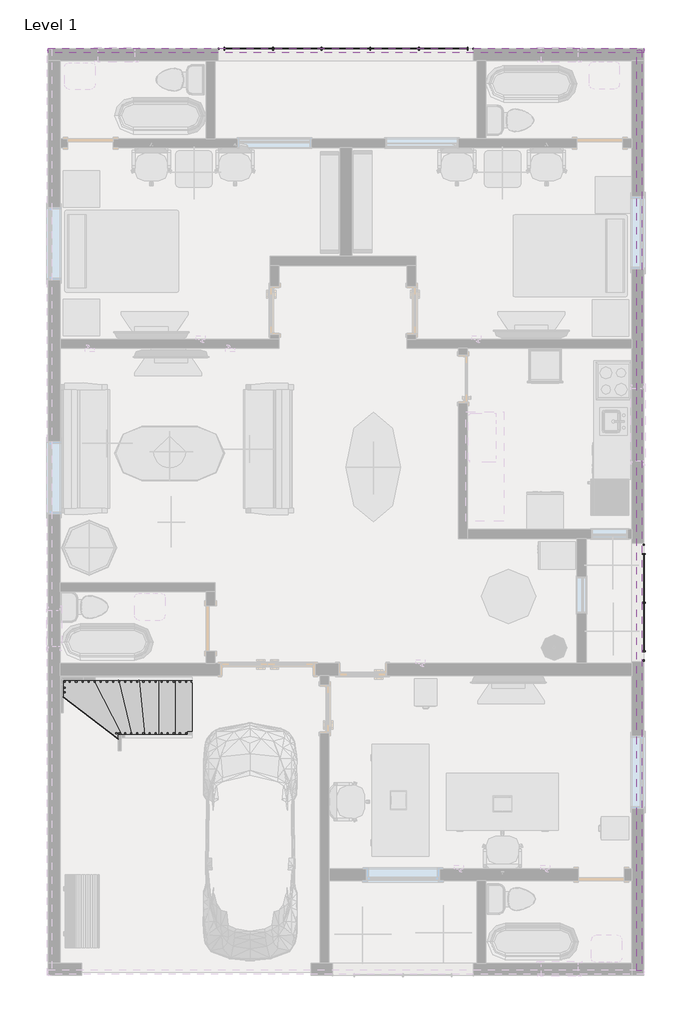
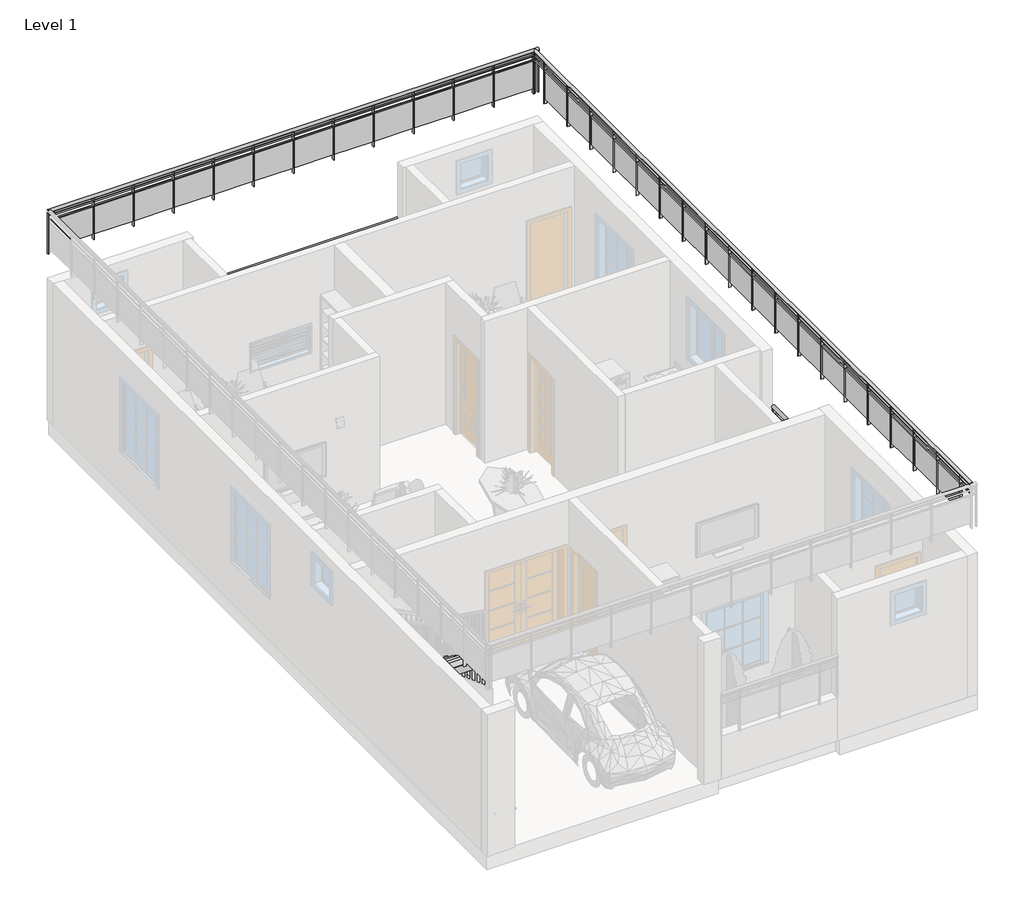
# One storey, part 4 of 5: 4 railings, 1 stair flight.
"""IFC4 building model written with IfcOpenShell, lengths in millimetres."""

from ifc_helpers import new_model, si_unit, point, frame, origin, place, context, project, spatial, polyline, ellipse_curve, trimmed, outline, extrude, transform, mapped, element, save
from ifc_brep_helpers import plane_surface, extruded_surface, advanced_brep
from components import stair_flight_393df7a1

model = new_model("IFC4")

# Units and contexts
model_context = context("Model", 3, world=origin())
ifc_project = project(units=[si_unit("LENGTHUNIT", "METRE", prefix="MILLI")], contexts=[model_context])

# Site, building, storey
site = spatial("IfcSite", under=ifc_project)
building = spatial("IfcBuilding", under=site)
storey = spatial("IfcBuildingStorey", under=building, Name="Level 1", Elevation=0.0)

# Railings
placement = place(None, origin())
element("IfcRailing", 1, ObjectType="Glass Panel - Bottom Fill", at=placement, inside=storey, context=model_context, shape_type="SolidModel", body=[
    advanced_brep(
    [(-4454.3957152, 16105.8691167, 1828.8), (-4454.3957152, 16029.6691167, 1828.8), (-187.1957152, 16105.8691167, 1828.8), (-187.1957152, 16029.6691167, 1828.8)],
    [
        (0, 1, ellipse_curve(frame((-4454.3957152, 16067.7691167, 1828.8), z_axis=(-1.0, 0.0, 0.0), x_axis=(0.0, -1.0, 0.0)), 38.1, 28.575)),
        (1, 0, ellipse_curve(frame((-4454.3957152, 16067.7691167, 1828.8), z_axis=(-1.0, 0.0, 0.0), x_axis=(0.0, -1.0, 0.0)), 38.1, 28.575)),
        (2, 3, ellipse_curve(frame((-187.1957152, 16067.7691167, 1828.8), z_axis=(1.0, 0.0, 0.0), x_axis=(0.0, -1.0, 0.0)), 38.1, 28.575)),
        (3, 2, ellipse_curve(frame((-187.1957152, 16067.7691167, 1828.8), z_axis=(1.0, 0.0, 0.0), x_axis=(0.0, -1.0, 0.0)), 38.1, 28.575)),
        (0, 2),
        (3, 1),
    ],
    [
        plane_surface(frame((-4454.3957152, 16067.7691167, 1828.8), z_axis=(-1.0, 0.0, 0.0), x_axis=(0.0, 1.0, 0.0))),
        plane_surface(frame((-187.1957152, 16067.7691167, 1828.8), z_axis=(1.0, 0.0, 0.0), x_axis=(0.0, 1.0, 0.0))),
        extruded_surface(trimmed(ellipse_curve(frame((-187.1957152, 16067.7691167, 1828.8), z_axis=(-1.0, 0.0, 0.0), x_axis=(0.0, -1.0, 0.0)), 38.1, 28.575), [point((-187.1957152, 16105.8691167, 1828.8))], [point((-187.1957152, 16029.6691167, 1828.8))], True, "CARTESIAN"), (-4267.200000000001, 0.0, 0.0), 4267.200000000001),
        extruded_surface(trimmed(ellipse_curve(frame((-187.1957152, 16067.7691167, 1828.8), z_axis=(-1.0, 0.0, 0.0), x_axis=(0.0, -1.0, 0.0)), 38.1, 28.575), [point((-187.1957152, 16029.6691167, 1828.8))], [point((-187.1957152, 16105.8691167, 1828.8))], True, "CARTESIAN"), (-4267.200000000001, 0.0, 0.0), 4267.200000000001),
    ],
    [
        (0, [[1, 2]]),
        (1, [[3, 4]]),
        (2, [[-1, 5, -4, 6]]),
        (3, [[-2, -6, -3, -5]]),
    ],
),
    extrude(outline(polyline([(-4454.3957152, 16055.0691167), (-4454.3957152, 16080.4691167), (-187.1957152, 16080.4691167), (-187.1957152, 16055.0691167), (-4454.3957152, 16055.0691167)])), frame((0.0, 0.0, 1714.5), z_axis=(0.0, 0.0, 1.0), x_axis=(1.0, 0.0, 0.0)), (0.0, 0.0, 1.0), 25.4),
    extrude(outline(polyline([(-4454.3957152, 16055.0691167), (-4454.3957152, 16080.4691167), (-187.1957152, 16080.4691167), (-187.1957152, 16055.0691167), (-4454.3957152, 16055.0691167)])), frame((0.0, 0.0, 1612.9), z_axis=(0.0, 0.0, 1.0), x_axis=(1.0, 0.0, 0.0)), (0.0, 0.0, 1.0), 25.4),
    extrude(outline(polyline([(-295.1457152, 16042.3691167), (-295.1457152, 16093.1691167), (-282.4457152, 16093.1691167), (-282.4457152, 16042.3691167), (-295.1457152, 16042.3691167)])), frame((0.0, 0.0, 914.4), z_axis=(0.0, 0.0, 1.0), x_axis=(1.0, 0.0, 0.0)), (0.0, 0.0, 1.0), 885.6788223),
    extrude(outline(polyline([(-1101.5957152, 16074.3042737), (-288.7957152, 16074.3042737), (-288.7957152, 16067.9542737), (-1101.5957152, 16067.9542737), (-1101.5957152, 16074.3042737)])), frame((0.0, 0.0, 1016.0), z_axis=(0.0, 0.0, 1.0), x_axis=(1.0, 0.0, 0.0)), (0.0, 0.0, 1.0), 596.9),
    extrude(outline(polyline([(-1107.9457152, 16042.3691167), (-1107.9457152, 16093.1691167), (-1095.2457152, 16093.1691167), (-1095.2457152, 16042.3691167), (-1107.9457152, 16042.3691167)])), frame((0.0, 0.0, 914.4), z_axis=(0.0, 0.0, 1.0), x_axis=(1.0, 0.0, 0.0)), (0.0, 0.0, 1.0), 885.6788223),
    extrude(outline(polyline([(-1914.3957152, 16074.3042737), (-1101.5957152, 16074.3042737), (-1101.5957152, 16067.9542737), (-1914.3957152, 16067.9542737), (-1914.3957152, 16074.3042737)])), frame((0.0, 0.0, 1016.0), z_axis=(0.0, 0.0, 1.0), x_axis=(1.0, 0.0, 0.0)), (0.0, 0.0, 1.0), 596.9),
    extrude(outline(polyline([(-1920.7457152, 16042.3691167), (-1920.7457152, 16093.1691167), (-1908.0457152, 16093.1691167), (-1908.0457152, 16042.3691167), (-1920.7457152, 16042.3691167)])), frame((0.0, 0.0, 914.4), z_axis=(0.0, 0.0, 1.0), x_axis=(1.0, 0.0, 0.0)), (0.0, 0.0, 1.0), 885.6788223),
    extrude(outline(polyline([(-2727.1957152, 16074.3042737), (-1914.3957152, 16074.3042737), (-1914.3957152, 16067.9542737), (-2727.1957152, 16067.9542737), (-2727.1957152, 16074.3042737)])), frame((0.0, 0.0, 1016.0), z_axis=(0.0, 0.0, 1.0), x_axis=(1.0, 0.0, 0.0)), (0.0, 0.0, 1.0), 596.9),
    extrude(outline(polyline([(-2733.5457152, 16042.3691167), (-2733.5457152, 16093.1691167), (-2720.8457152, 16093.1691167), (-2720.8457152, 16042.3691167), (-2733.5457152, 16042.3691167)])), frame((0.0, 0.0, 914.4), z_axis=(0.0, 0.0, 1.0), x_axis=(1.0, 0.0, 0.0)), (0.0, 0.0, 1.0), 885.6788223),
    extrude(outline(polyline([(-3539.9957152, 16074.3042737), (-2727.1957152, 16074.3042737), (-2727.1957152, 16067.9542737), (-3539.9957152, 16067.9542737), (-3539.9957152, 16074.3042737)])), frame((0.0, 0.0, 1016.0), z_axis=(0.0, 0.0, 1.0), x_axis=(1.0, 0.0, 0.0)), (0.0, 0.0, 1.0), 596.9),
    extrude(outline(polyline([(-3546.3457152, 16042.3691167), (-3546.3457152, 16093.1691167), (-3533.6457152, 16093.1691167), (-3533.6457152, 16042.3691167), (-3546.3457152, 16042.3691167)])), frame((0.0, 0.0, 914.4), z_axis=(0.0, 0.0, 1.0), x_axis=(1.0, 0.0, 0.0)), (0.0, 0.0, 1.0), 885.6788223),
    extrude(outline(polyline([(-4352.7957152, 16074.3042737), (-3539.9957152, 16074.3042737), (-3539.9957152, 16067.9542737), (-4352.7957152, 16067.9542737), (-4352.7957152, 16074.3042737)])), frame((0.0, 0.0, 1016.0), z_axis=(0.0, 0.0, 1.0), x_axis=(1.0, 0.0, 0.0)), (0.0, 0.0, 1.0), 596.9),
    extrude(outline(polyline([(-4359.1457152, 16042.3691167), (-4359.1457152, 16093.1691167), (-4346.4457152, 16093.1691167), (-4346.4457152, 16042.3691167), (-4359.1457152, 16042.3691167)])), frame((0.0, 0.0, 914.4), z_axis=(0.0, 0.0, 1.0), x_axis=(1.0, 0.0, 0.0)), (0.0, 0.0, 1.0), 885.6788223),
    extrude(outline(polyline([(-199.8957152, 16058.2441167), (-199.8957152, 16077.2941167), (-180.8457152, 16077.2941167), (-180.8457152, 16058.2441167), (-199.8957152, 16058.2441167)])), frame((0.0, 0.0, 914.4), z_axis=(0.0, 0.0, 1.0), x_axis=(1.0, 0.0, 0.0)), (0.0, 0.0, 1.0), 885.6788223),
    extrude(outline(polyline([(-4460.7457152, 16058.2441167), (-4460.7457152, 16077.2941167), (-4441.6957152, 16077.2941167), (-4441.6957152, 16058.2441167), (-4460.7457152, 16058.2441167)])), frame((0.0, 0.0, 914.4), z_axis=(0.0, 0.0, 1.0), x_axis=(1.0, 0.0, 0.0)), (0.0, 0.0, 1.0), 885.6788223),
])
element("IfcRailing", 2, ObjectType="Glass Panel - Bottom Fill", at=placement, inside=storey, context=model_context, shape_type="SolidModel", body=[
    advanced_brep(
    [(2695.7042848, 7787.3691167, 1828.8), (2619.5042848, 7787.3691167, 1828.8), (2695.7042848, 5850.6191167, 1828.8), (2619.5042848, 5850.6191167, 1828.8)],
    [
        (0, 1, ellipse_curve(frame((2657.6042848, 7787.3691167, 1828.8), z_axis=(0.0, 1.0, 0.0), x_axis=(-1.0, 0.0, 0.0)), 38.1, 28.575)),
        (1, 0, ellipse_curve(frame((2657.6042848, 7787.3691167, 1828.8), z_axis=(0.0, 1.0, 0.0), x_axis=(-1.0, 0.0, 0.0)), 38.1, 28.575)),
        (2, 3, ellipse_curve(frame((2657.6042848, 5850.6191167, 1828.8), z_axis=(0.0, -1.0, 0.0), x_axis=(-1.0, 0.0, 0.0)), 38.1, 28.575)),
        (3, 2, ellipse_curve(frame((2657.6042848, 5850.6191167, 1828.8), z_axis=(0.0, -1.0, 0.0), x_axis=(-1.0, 0.0, 0.0)), 38.1, 28.575)),
        (0, 2),
        (3, 1),
    ],
    [
        plane_surface(frame((2657.6042848, 7787.3691167, 1828.8), z_axis=(0.0, 1.0, 0.0), x_axis=(0.0, 0.0, -1.0))),
        plane_surface(frame((2657.6042848, 5850.6191167, 1828.8), z_axis=(0.0, -1.0, 0.0), x_axis=(0.0, 0.0, -1.0))),
        extruded_surface(trimmed(ellipse_curve(frame((2657.6042848, 5850.6191167, 1828.8), z_axis=(0.0, 1.0, 0.0), x_axis=(-1.0, 0.0, 0.0)), 38.1, 28.575), [point((2695.7042848, 5850.6191167, 1828.8))], [point((2619.5042848, 5850.6191167, 1828.8))], True, "CARTESIAN"), (0.0, 1936.75, 0.0), 1936.75),
        extruded_surface(trimmed(ellipse_curve(frame((2657.6042848, 5850.6191167, 1828.8), z_axis=(0.0, 1.0, 0.0), x_axis=(-1.0, 0.0, 0.0)), 38.1, 28.575), [point((2619.5042848, 5850.6191167, 1828.8))], [point((2695.7042848, 5850.6191167, 1828.8))], True, "CARTESIAN"), (0.0, 1936.75, 0.0), 1936.75),
    ],
    [
        (0, [[1, 2]]),
        (1, [[3, 4]]),
        (2, [[-1, 5, -4, 6]]),
        (3, [[-2, -6, -3, -5]]),
    ],
),
    extrude(outline(polyline([(2644.9042848, 7787.3691167), (2670.3042848, 7787.3691167), (2670.3042848, 5850.6191167), (2644.9042848, 5850.6191167), (2644.9042848, 7787.3691167)])), frame((0.0, 0.0, 1714.5), z_axis=(0.0, 0.0, 1.0), x_axis=(1.0, 0.0, 0.0)), (0.0, 0.0, 1.0), 25.4),
    extrude(outline(polyline([(2644.9042848, 7787.3691167), (2670.3042848, 7787.3691167), (2670.3042848, 5850.6191167), (2644.9042848, 5850.6191167), (2644.9042848, 7787.3691167)])), frame((0.0, 0.0, 1612.9), z_axis=(0.0, 0.0, 1.0), x_axis=(1.0, 0.0, 0.0)), (0.0, 0.0, 1.0), 25.4),
    extrude(outline(polyline([(2632.2042848, 6012.5441167), (2683.0042848, 6012.5441167), (2683.0042848, 5999.8441167), (2632.2042848, 5999.8441167), (2632.2042848, 6012.5441167)])), frame((0.0, 0.0, 914.4), z_axis=(0.0, 0.0, 1.0), x_axis=(1.0, 0.0, 0.0)), (0.0, 0.0, 1.0), 885.6788223),
    extrude(outline(polyline([(2664.1394419, 6818.9941167), (2664.1394419, 6006.1941167), (2657.7894419, 6006.1941167), (2657.7894419, 6818.9941167), (2664.1394419, 6818.9941167)])), frame((0.0, 0.0, 1016.0), z_axis=(0.0, 0.0, 1.0), x_axis=(1.0, 0.0, 0.0)), (0.0, 0.0, 1.0), 596.9),
    extrude(outline(polyline([(2632.2042848, 6825.3441167), (2683.0042848, 6825.3441167), (2683.0042848, 6812.6441167), (2632.2042848, 6812.6441167), (2632.2042848, 6825.3441167)])), frame((0.0, 0.0, 914.4), z_axis=(0.0, 0.0, 1.0), x_axis=(1.0, 0.0, 0.0)), (0.0, 0.0, 1.0), 885.6788223),
    extrude(outline(polyline([(2664.1394419, 7631.7941167), (2664.1394419, 6818.9941167), (2657.7894419, 6818.9941167), (2657.7894419, 7631.7941167), (2664.1394419, 7631.7941167)])), frame((0.0, 0.0, 1016.0), z_axis=(0.0, 0.0, 1.0), x_axis=(1.0, 0.0, 0.0)), (0.0, 0.0, 1.0), 596.9),
    extrude(outline(polyline([(2632.2042848, 7638.1441167), (2683.0042848, 7638.1441167), (2683.0042848, 7625.4441167), (2632.2042848, 7625.4441167), (2632.2042848, 7638.1441167)])), frame((0.0, 0.0, 914.4), z_axis=(0.0, 0.0, 1.0), x_axis=(1.0, 0.0, 0.0)), (0.0, 0.0, 1.0), 885.6788223),
    extrude(outline(polyline([(2648.0792848, 5863.3191167), (2667.1292848, 5863.3191167), (2667.1292848, 5844.2691167), (2648.0792848, 5844.2691167), (2648.0792848, 5863.3191167)])), frame((0.0, 0.0, 914.4), z_axis=(0.0, 0.0, 1.0), x_axis=(1.0, 0.0, 0.0)), (0.0, 0.0, 1.0), 885.6788223),
    extrude(outline(polyline([(2648.0792848, 7793.7191167), (2667.1292848, 7793.7191167), (2667.1292848, 7774.6691167), (2648.0792848, 7774.6691167), (2648.0792848, 7793.7191167)])), frame((0.0, 0.0, 914.4), z_axis=(0.0, 0.0, 1.0), x_axis=(1.0, 0.0, 0.0)), (0.0, 0.0, 1.0), 885.6788223),
])
element("IfcRailing", 3, ObjectType="Glass Panel - Bottom Fill", at=placement, inside=storey, context=model_context, shape_type="SolidModel", body=[
    advanced_brep(
    [(-7299.1957152, 16080.4691167, 4495.8), (-7299.1957152, 16004.2691167, 4495.8), (2657.6042848, 16080.4691167, 4495.8), (2657.6042848, 16004.2691167, 4495.8)],
    [
        (0, 1, ellipse_curve(frame((-7299.1957152, 16042.3691167, 4495.8), z_axis=(-1.0, 0.0, 0.0), x_axis=(0.0, -1.0, 0.0)), 38.1, 28.575)),
        (1, 0, ellipse_curve(frame((-7299.1957152, 16042.3691167, 4495.8), z_axis=(-1.0, 0.0, 0.0), x_axis=(0.0, -1.0, 0.0)), 38.1, 28.575)),
        (2, 3, ellipse_curve(frame((2657.6042848, 16042.3691167, 4495.8), z_axis=(1.0, 0.0, 0.0), x_axis=(0.0, -1.0, 0.0)), 38.1, 28.575)),
        (3, 2, ellipse_curve(frame((2657.6042848, 16042.3691167, 4495.8), z_axis=(1.0, 0.0, 0.0), x_axis=(0.0, -1.0, 0.0)), 38.1, 28.575)),
        (0, 2),
        (3, 1),
    ],
    [
        plane_surface(frame((-7299.1957152, 16042.3691167, 4495.8), z_axis=(-1.0, 0.0, 0.0), x_axis=(0.0, 1.0, 0.0))),
        plane_surface(frame((2657.6042848, 16042.3691167, 4495.8), z_axis=(1.0, 0.0, 0.0), x_axis=(0.0, 1.0, 0.0))),
        extruded_surface(trimmed(ellipse_curve(frame((2657.6042848, 16042.3691167, 4495.8), z_axis=(-1.0, 0.0, 0.0), x_axis=(0.0, -1.0, 0.0)), 38.1, 28.575), [point((2657.6042848, 16080.4691167, 4495.8))], [point((2657.6042848, 16004.2691167, 4495.8))], True, "CARTESIAN"), (-9956.800000000001, 0.0, 0.0), 9956.800000000001),
        extruded_surface(trimmed(ellipse_curve(frame((2657.6042848, 16042.3691167, 4495.8), z_axis=(-1.0, 0.0, 0.0), x_axis=(0.0, -1.0, 0.0)), 38.1, 28.575), [point((2657.6042848, 16004.2691167, 4495.8))], [point((2657.6042848, 16080.4691167, 4495.8))], True, "CARTESIAN"), (-9956.800000000001, 0.0, 0.0), 9956.800000000001),
    ],
    [
        (0, [[1, 2]]),
        (1, [[3, 4]]),
        (2, [[-1, 5, -4, 6]]),
        (3, [[-2, -6, -3, -5]]),
    ],
),
    extrude(outline(polyline([(-7299.1957152, 16029.6691167), (-7299.1957152, 16055.0691167), (2657.6042848, 16055.0691167), (2657.6042848, 16029.6691167), (-7299.1957152, 16029.6691167)])), frame((0.0, 0.0, 4381.5), z_axis=(0.0, 0.0, 1.0), x_axis=(1.0, 0.0, 0.0)), (0.0, 0.0, 1.0), 25.4),
    extrude(outline(polyline([(-7299.1957152, 16029.6691167), (-7299.1957152, 16055.0691167), (2657.6042848, 16055.0691167), (2657.6042848, 16029.6691167), (-7299.1957152, 16029.6691167)])), frame((0.0, 0.0, 4279.9), z_axis=(0.0, 0.0, 1.0), x_axis=(1.0, 0.0, 0.0)), (0.0, 0.0, 1.0), 25.4),
    extrude(outline(polyline([(2549.6542848, 16016.9691167), (2549.6542848, 16067.7691167), (2562.3542848, 16067.7691167), (2562.3542848, 16016.9691167), (2549.6542848, 16016.9691167)])), frame((0.0, 0.0, 3581.4), z_axis=(0.0, 0.0, 1.0), x_axis=(1.0, 0.0, 0.0)), (0.0, 0.0, 1.0), 885.6788223),
    extrude(outline(polyline([(1743.2042848, 16048.9042737), (2556.0042848, 16048.9042737), (2556.0042848, 16042.5542737), (1743.2042848, 16042.5542737), (1743.2042848, 16048.9042737)])), frame((0.0, 0.0, 3683.0), z_axis=(0.0, 0.0, 1.0), x_axis=(1.0, 0.0, 0.0)), (0.0, 0.0, 1.0), 596.9),
    extrude(outline(polyline([(1736.8542848, 16016.9691167), (1736.8542848, 16067.7691167), (1749.5542848, 16067.7691167), (1749.5542848, 16016.9691167), (1736.8542848, 16016.9691167)])), frame((0.0, 0.0, 3581.4), z_axis=(0.0, 0.0, 1.0), x_axis=(1.0, 0.0, 0.0)), (0.0, 0.0, 1.0), 885.6788223),
    extrude(outline(polyline([(930.4042848, 16048.9042737), (1743.2042848, 16048.9042737), (1743.2042848, 16042.5542737), (930.4042848, 16042.5542737), (930.4042848, 16048.9042737)])), frame((0.0, 0.0, 3683.0), z_axis=(0.0, 0.0, 1.0), x_axis=(1.0, 0.0, 0.0)), (0.0, 0.0, 1.0), 596.9),
    extrude(outline(polyline([(924.0542848, 16016.9691167), (924.0542848, 16067.7691167), (936.7542848, 16067.7691167), (936.7542848, 16016.9691167), (924.0542848, 16016.9691167)])), frame((0.0, 0.0, 3581.4), z_axis=(0.0, 0.0, 1.0), x_axis=(1.0, 0.0, 0.0)), (0.0, 0.0, 1.0), 885.6788223),
    extrude(outline(polyline([(117.6042848, 16048.9042737), (930.4042848, 16048.9042737), (930.4042848, 16042.5542737), (117.6042848, 16042.5542737), (117.6042848, 16048.9042737)])), frame((0.0, 0.0, 3683.0), z_axis=(0.0, 0.0, 1.0), x_axis=(1.0, 0.0, 0.0)), (0.0, 0.0, 1.0), 596.9),
    extrude(outline(polyline([(111.2542848, 16016.9691167), (111.2542848, 16067.7691167), (123.9542848, 16067.7691167), (123.9542848, 16016.9691167), (111.2542848, 16016.9691167)])), frame((0.0, 0.0, 3581.4), z_axis=(0.0, 0.0, 1.0), x_axis=(1.0, 0.0, 0.0)), (0.0, 0.0, 1.0), 885.6788223),
    extrude(outline(polyline([(-695.1957152, 16048.9042737), (117.6042848, 16048.9042737), (117.6042848, 16042.5542737), (-695.1957152, 16042.5542737), (-695.1957152, 16048.9042737)])), frame((0.0, 0.0, 3683.0), z_axis=(0.0, 0.0, 1.0), x_axis=(1.0, 0.0, 0.0)), (0.0, 0.0, 1.0), 596.9),
    extrude(outline(polyline([(-701.5457152, 16016.9691167), (-701.5457152, 16067.7691167), (-688.8457152, 16067.7691167), (-688.8457152, 16016.9691167), (-701.5457152, 16016.9691167)])), frame((0.0, 0.0, 3581.4), z_axis=(0.0, 0.0, 1.0), x_axis=(1.0, 0.0, 0.0)), (0.0, 0.0, 1.0), 885.6788223),
    extrude(outline(polyline([(-1507.9957152, 16048.9042737), (-695.1957152, 16048.9042737), (-695.1957152, 16042.5542737), (-1507.9957152, 16042.5542737), (-1507.9957152, 16048.9042737)])), frame((0.0, 0.0, 3683.0), z_axis=(0.0, 0.0, 1.0), x_axis=(1.0, 0.0, 0.0)), (0.0, 0.0, 1.0), 596.9),
    extrude(outline(polyline([(-1514.3457152, 16016.9691167), (-1514.3457152, 16067.7691167), (-1501.6457152, 16067.7691167), (-1501.6457152, 16016.9691167), (-1514.3457152, 16016.9691167)])), frame((0.0, 0.0, 3581.4), z_axis=(0.0, 0.0, 1.0), x_axis=(1.0, 0.0, 0.0)), (0.0, 0.0, 1.0), 885.6788223),
    extrude(outline(polyline([(-2320.7957152, 16048.9042737), (-1507.9957152, 16048.9042737), (-1507.9957152, 16042.5542737), (-2320.7957152, 16042.5542737), (-2320.7957152, 16048.9042737)])), frame((0.0, 0.0, 3683.0), z_axis=(0.0, 0.0, 1.0), x_axis=(1.0, 0.0, 0.0)), (0.0, 0.0, 1.0), 596.9),
    extrude(outline(polyline([(-2327.1457152, 16016.9691167), (-2327.1457152, 16067.7691167), (-2314.4457152, 16067.7691167), (-2314.4457152, 16016.9691167), (-2327.1457152, 16016.9691167)])), frame((0.0, 0.0, 3581.4), z_axis=(0.0, 0.0, 1.0), x_axis=(1.0, 0.0, 0.0)), (0.0, 0.0, 1.0), 885.6788223),
    extrude(outline(polyline([(-3133.5957152, 16048.9042737), (-2320.7957152, 16048.9042737), (-2320.7957152, 16042.5542737), (-3133.5957152, 16042.5542737), (-3133.5957152, 16048.9042737)])), frame((0.0, 0.0, 3683.0), z_axis=(0.0, 0.0, 1.0), x_axis=(1.0, 0.0, 0.0)), (0.0, 0.0, 1.0), 596.9),
    extrude(outline(polyline([(-3139.9457152, 16016.9691167), (-3139.9457152, 16067.7691167), (-3127.2457152, 16067.7691167), (-3127.2457152, 16016.9691167), (-3139.9457152, 16016.9691167)])), frame((0.0, 0.0, 3581.4), z_axis=(0.0, 0.0, 1.0), x_axis=(1.0, 0.0, 0.0)), (0.0, 0.0, 1.0), 885.6788223),
    extrude(outline(polyline([(-3946.3957152, 16048.9042737), (-3133.5957152, 16048.9042737), (-3133.5957152, 16042.5542737), (-3946.3957152, 16042.5542737), (-3946.3957152, 16048.9042737)])), frame((0.0, 0.0, 3683.0), z_axis=(0.0, 0.0, 1.0), x_axis=(1.0, 0.0, 0.0)), (0.0, 0.0, 1.0), 596.9),
    extrude(outline(polyline([(-3952.7457152, 16016.9691167), (-3952.7457152, 16067.7691167), (-3940.0457152, 16067.7691167), (-3940.0457152, 16016.9691167), (-3952.7457152, 16016.9691167)])), frame((0.0, 0.0, 3581.4), z_axis=(0.0, 0.0, 1.0), x_axis=(1.0, 0.0, 0.0)), (0.0, 0.0, 1.0), 885.6788223),
    extrude(outline(polyline([(-4759.1957152, 16048.9042737), (-3946.3957152, 16048.9042737), (-3946.3957152, 16042.5542737), (-4759.1957152, 16042.5542737), (-4759.1957152, 16048.9042737)])), frame((0.0, 0.0, 3683.0), z_axis=(0.0, 0.0, 1.0), x_axis=(1.0, 0.0, 0.0)), (0.0, 0.0, 1.0), 596.9),
    extrude(outline(polyline([(-4765.5457152, 16016.9691167), (-4765.5457152, 16067.7691167), (-4752.8457152, 16067.7691167), (-4752.8457152, 16016.9691167), (-4765.5457152, 16016.9691167)])), frame((0.0, 0.0, 3581.4), z_axis=(0.0, 0.0, 1.0), x_axis=(1.0, 0.0, 0.0)), (0.0, 0.0, 1.0), 885.6788223),
    extrude(outline(polyline([(-5571.9957152, 16048.9042737), (-4759.1957152, 16048.9042737), (-4759.1957152, 16042.5542737), (-5571.9957152, 16042.5542737), (-5571.9957152, 16048.9042737)])), frame((0.0, 0.0, 3683.0), z_axis=(0.0, 0.0, 1.0), x_axis=(1.0, 0.0, 0.0)), (0.0, 0.0, 1.0), 596.9),
    extrude(outline(polyline([(-5578.3457152, 16016.9691167), (-5578.3457152, 16067.7691167), (-5565.6457152, 16067.7691167), (-5565.6457152, 16016.9691167), (-5578.3457152, 16016.9691167)])), frame((0.0, 0.0, 3581.4), z_axis=(0.0, 0.0, 1.0), x_axis=(1.0, 0.0, 0.0)), (0.0, 0.0, 1.0), 885.6788223),
    extrude(outline(polyline([(-6384.7957152, 16048.9042737), (-5571.9957152, 16048.9042737), (-5571.9957152, 16042.5542737), (-6384.7957152, 16042.5542737), (-6384.7957152, 16048.9042737)])), frame((0.0, 0.0, 3683.0), z_axis=(0.0, 0.0, 1.0), x_axis=(1.0, 0.0, 0.0)), (0.0, 0.0, 1.0), 596.9),
    extrude(outline(polyline([(-6391.1457152, 16016.9691167), (-6391.1457152, 16067.7691167), (-6378.4457152, 16067.7691167), (-6378.4457152, 16016.9691167), (-6391.1457152, 16016.9691167)])), frame((0.0, 0.0, 3581.4), z_axis=(0.0, 0.0, 1.0), x_axis=(1.0, 0.0, 0.0)), (0.0, 0.0, 1.0), 885.6788223),
    extrude(outline(polyline([(-7197.5957152, 16048.9042737), (-6384.7957152, 16048.9042737), (-6384.7957152, 16042.5542737), (-7197.5957152, 16042.5542737), (-7197.5957152, 16048.9042737)])), frame((0.0, 0.0, 3683.0), z_axis=(0.0, 0.0, 1.0), x_axis=(1.0, 0.0, 0.0)), (0.0, 0.0, 1.0), 596.9),
    extrude(outline(polyline([(-7203.9457152, 16016.9691167), (-7203.9457152, 16067.7691167), (-7191.2457152, 16067.7691167), (-7191.2457152, 16016.9691167), (-7203.9457152, 16016.9691167)])), frame((0.0, 0.0, 3581.4), z_axis=(0.0, 0.0, 1.0), x_axis=(1.0, 0.0, 0.0)), (0.0, 0.0, 1.0), 885.6788223),
    extrude(outline(polyline([(2644.9042848, 16032.8441167), (2644.9042848, 16051.8941167), (2663.9542848, 16051.8941167), (2663.9542848, 16032.8441167), (2644.9042848, 16032.8441167)])), frame((0.0, 0.0, 3581.4), z_axis=(0.0, 0.0, 1.0), x_axis=(1.0, 0.0, 0.0)), (0.0, 0.0, 1.0), 885.6788223),
    extrude(outline(polyline([(-7305.5457152, 16032.8441167), (-7305.5457152, 16051.8941167), (-7286.4957152, 16051.8941167), (-7286.4957152, 16032.8441167), (-7305.5457152, 16032.8441167)])), frame((0.0, 0.0, 3581.4), z_axis=(0.0, 0.0, 1.0), x_axis=(1.0, 0.0, 0.0)), (0.0, 0.0, 1.0), 885.6788223),
])
element("IfcRailing", 4, ObjectType="Glass Panel - Bottom Fill", at=placement, inside=storey, context=model_context, shape_type="SolidModel", body=[
    advanced_brep(
    [(2543.3042848, 675.3691167, 4495.8), (2619.5042848, 675.3691167, 4495.8), (2543.3042848, 16042.3691167, 4495.8), (2619.5042848, 16042.3691167, 4495.8)],
    [
        (0, 1, ellipse_curve(frame((2581.4042848, 675.3691167, 4495.8), z_axis=(0.0, -1.0, 0.0), x_axis=(1.0, 0.0, 0.0)), 38.1, 28.575)),
        (1, 0, ellipse_curve(frame((2581.4042848, 675.3691167, 4495.8), z_axis=(0.0, -1.0, 0.0), x_axis=(1.0, 0.0, 0.0)), 38.1, 28.575)),
        (2, 3, ellipse_curve(frame((2581.4042848, 16042.3691167, 4495.8), z_axis=(0.0, 1.0, 0.0), x_axis=(1.0, 0.0, 0.0)), 38.1, 28.575)),
        (3, 2, ellipse_curve(frame((2581.4042848, 16042.3691167, 4495.8), z_axis=(0.0, 1.0, 0.0), x_axis=(1.0, 0.0, 0.0)), 38.1, 28.575)),
        (0, 2),
        (3, 1),
    ],
    [
        plane_surface(frame((2581.4042848, 675.3691167, 4495.8), z_axis=(0.0, -1.0, 0.0), x_axis=(0.0, 0.0, 1.0))),
        plane_surface(frame((2581.4042848, 16042.3691167, 4495.8), z_axis=(0.0, 1.0, 0.0), x_axis=(0.0, 0.0, 1.0))),
        extruded_surface(trimmed(ellipse_curve(frame((2581.4042848, 16042.3691167, 4495.8), z_axis=(0.0, -1.0, 0.0), x_axis=(1.0, 0.0, 0.0)), 38.1, 28.575), [point((2543.3042848, 16042.3691167, 4495.8))], [point((2619.5042848, 16042.3691167, 4495.8))], True, "CARTESIAN"), (0.0, -15367.0, 0.0), 15367.0),
        extruded_surface(trimmed(ellipse_curve(frame((2581.4042848, 16042.3691167, 4495.8), z_axis=(0.0, -1.0, 0.0), x_axis=(1.0, 0.0, 0.0)), 38.1, 28.575), [point((2619.5042848, 16042.3691167, 4495.8))], [point((2543.3042848, 16042.3691167, 4495.8))], True, "CARTESIAN"), (0.0, -15367.0, 0.0), 15367.0),
    ],
    [
        (0, [[1, 2]]),
        (1, [[3, 4]]),
        (2, [[-1, 5, -4, 6]]),
        (3, [[-2, -6, -3, -5]]),
    ],
),
    extrude(outline(polyline([(2594.1042848, 675.3691167), (2568.7042848, 675.3691167), (2568.7042848, 16042.3691167), (2594.1042848, 16042.3691167), (2594.1042848, 675.3691167)])), frame((0.0, 0.0, 4381.5), z_axis=(0.0, 0.0, 1.0), x_axis=(1.0, 0.0, 0.0)), (0.0, 0.0, 1.0), 25.4),
    extrude(outline(polyline([(2594.1042848, 675.3691167), (2568.7042848, 675.3691167), (2568.7042848, 16042.3691167), (2594.1042848, 16042.3691167), (2594.1042848, 675.3691167)])), frame((0.0, 0.0, 4279.9), z_axis=(0.0, 0.0, 1.0), x_axis=(1.0, 0.0, 0.0)), (0.0, 0.0, 1.0), 25.4),
    extrude(outline(polyline([(2606.8042848, 15667.7191167), (2556.0042848, 15667.7191167), (2556.0042848, 15680.4191167), (2606.8042848, 15680.4191167), (2606.8042848, 15667.7191167)])), frame((0.0, 0.0, 3581.4), z_axis=(0.0, 0.0, 1.0), x_axis=(1.0, 0.0, 0.0)), (0.0, 0.0, 1.0), 885.6788223),
    extrude(outline(polyline([(2574.8691278, 14861.2691167), (2574.8691278, 15674.0691167), (2581.2191278, 15674.0691167), (2581.2191278, 14861.2691167), (2574.8691278, 14861.2691167)])), frame((0.0, 0.0, 3683.0), z_axis=(0.0, 0.0, 1.0), x_axis=(1.0, 0.0, 0.0)), (0.0, 0.0, 1.0), 596.9),
    extrude(outline(polyline([(2606.8042848, 14854.9191167), (2556.0042848, 14854.9191167), (2556.0042848, 14867.6191167), (2606.8042848, 14867.6191167), (2606.8042848, 14854.9191167)])), frame((0.0, 0.0, 3581.4), z_axis=(0.0, 0.0, 1.0), x_axis=(1.0, 0.0, 0.0)), (0.0, 0.0, 1.0), 885.6788223),
    extrude(outline(polyline([(2574.8691278, 14048.4691167), (2574.8691278, 14861.2691167), (2581.2191278, 14861.2691167), (2581.2191278, 14048.4691167), (2574.8691278, 14048.4691167)])), frame((0.0, 0.0, 3683.0), z_axis=(0.0, 0.0, 1.0), x_axis=(1.0, 0.0, 0.0)), (0.0, 0.0, 1.0), 596.9),
    extrude(outline(polyline([(2606.8042848, 14042.1191167), (2556.0042848, 14042.1191167), (2556.0042848, 14054.8191167), (2606.8042848, 14054.8191167), (2606.8042848, 14042.1191167)])), frame((0.0, 0.0, 3581.4), z_axis=(0.0, 0.0, 1.0), x_axis=(1.0, 0.0, 0.0)), (0.0, 0.0, 1.0), 885.6788223),
    extrude(outline(polyline([(2574.8691278, 13235.6691167), (2574.8691278, 14048.4691167), (2581.2191278, 14048.4691167), (2581.2191278, 13235.6691167), (2574.8691278, 13235.6691167)])), frame((0.0, 0.0, 3683.0), z_axis=(0.0, 0.0, 1.0), x_axis=(1.0, 0.0, 0.0)), (0.0, 0.0, 1.0), 596.9),
    extrude(outline(polyline([(2606.8042848, 13229.3191167), (2556.0042848, 13229.3191167), (2556.0042848, 13242.0191167), (2606.8042848, 13242.0191167), (2606.8042848, 13229.3191167)])), frame((0.0, 0.0, 3581.4), z_axis=(0.0, 0.0, 1.0), x_axis=(1.0, 0.0, 0.0)), (0.0, 0.0, 1.0), 885.6788223),
    extrude(outline(polyline([(2574.8691278, 12422.8691167), (2574.8691278, 13235.6691167), (2581.2191278, 13235.6691167), (2581.2191278, 12422.8691167), (2574.8691278, 12422.8691167)])), frame((0.0, 0.0, 3683.0), z_axis=(0.0, 0.0, 1.0), x_axis=(1.0, 0.0, 0.0)), (0.0, 0.0, 1.0), 596.9),
    extrude(outline(polyline([(2606.8042848, 12416.5191167), (2556.0042848, 12416.5191167), (2556.0042848, 12429.2191167), (2606.8042848, 12429.2191167), (2606.8042848, 12416.5191167)])), frame((0.0, 0.0, 3581.4), z_axis=(0.0, 0.0, 1.0), x_axis=(1.0, 0.0, 0.0)), (0.0, 0.0, 1.0), 885.6788223),
    extrude(outline(polyline([(2574.8691278, 11610.0691167), (2574.8691278, 12422.8691167), (2581.2191278, 12422.8691167), (2581.2191278, 11610.0691167), (2574.8691278, 11610.0691167)])), frame((0.0, 0.0, 3683.0), z_axis=(0.0, 0.0, 1.0), x_axis=(1.0, 0.0, 0.0)), (0.0, 0.0, 1.0), 596.9),
    extrude(outline(polyline([(2606.8042848, 11603.7191167), (2556.0042848, 11603.7191167), (2556.0042848, 11616.4191167), (2606.8042848, 11616.4191167), (2606.8042848, 11603.7191167)])), frame((0.0, 0.0, 3581.4), z_axis=(0.0, 0.0, 1.0), x_axis=(1.0, 0.0, 0.0)), (0.0, 0.0, 1.0), 885.6788223),
    extrude(outline(polyline([(2574.8691278, 10797.2691167), (2574.8691278, 11610.0691167), (2581.2191278, 11610.0691167), (2581.2191278, 10797.2691167), (2574.8691278, 10797.2691167)])), frame((0.0, 0.0, 3683.0), z_axis=(0.0, 0.0, 1.0), x_axis=(1.0, 0.0, 0.0)), (0.0, 0.0, 1.0), 596.9),
    extrude(outline(polyline([(2606.8042848, 10790.9191167), (2556.0042848, 10790.9191167), (2556.0042848, 10803.6191167), (2606.8042848, 10803.6191167), (2606.8042848, 10790.9191167)])), frame((0.0, 0.0, 3581.4), z_axis=(0.0, 0.0, 1.0), x_axis=(1.0, 0.0, 0.0)), (0.0, 0.0, 1.0), 885.6788223),
    extrude(outline(polyline([(2574.8691278, 9984.4691167), (2574.8691278, 10797.2691167), (2581.2191278, 10797.2691167), (2581.2191278, 9984.4691167), (2574.8691278, 9984.4691167)])), frame((0.0, 0.0, 3683.0), z_axis=(0.0, 0.0, 1.0), x_axis=(1.0, 0.0, 0.0)), (0.0, 0.0, 1.0), 596.9),
    extrude(outline(polyline([(2606.8042848, 9978.1191167), (2556.0042848, 9978.1191167), (2556.0042848, 9990.8191167), (2606.8042848, 9990.8191167), (2606.8042848, 9978.1191167)])), frame((0.0, 0.0, 3581.4), z_axis=(0.0, 0.0, 1.0), x_axis=(1.0, 0.0, 0.0)), (0.0, 0.0, 1.0), 885.6788223),
    extrude(outline(polyline([(2574.8691278, 9171.6691167), (2574.8691278, 9984.4691167), (2581.2191278, 9984.4691167), (2581.2191278, 9171.6691167), (2574.8691278, 9171.6691167)])), frame((0.0, 0.0, 3683.0), z_axis=(0.0, 0.0, 1.0), x_axis=(1.0, 0.0, 0.0)), (0.0, 0.0, 1.0), 596.9),
    extrude(outline(polyline([(2606.8042848, 9165.3191167), (2556.0042848, 9165.3191167), (2556.0042848, 9178.0191167), (2606.8042848, 9178.0191167), (2606.8042848, 9165.3191167)])), frame((0.0, 0.0, 3581.4), z_axis=(0.0, 0.0, 1.0), x_axis=(1.0, 0.0, 0.0)), (0.0, 0.0, 1.0), 885.6788223),
    extrude(outline(polyline([(2574.8691278, 8358.8691167), (2574.8691278, 9171.6691167), (2581.2191278, 9171.6691167), (2581.2191278, 8358.8691167), (2574.8691278, 8358.8691167)])), frame((0.0, 0.0, 3683.0), z_axis=(0.0, 0.0, 1.0), x_axis=(1.0, 0.0, 0.0)), (0.0, 0.0, 1.0), 596.9),
    extrude(outline(polyline([(2606.8042848, 8352.5191167), (2556.0042848, 8352.5191167), (2556.0042848, 8365.2191167), (2606.8042848, 8365.2191167), (2606.8042848, 8352.5191167)])), frame((0.0, 0.0, 3581.4), z_axis=(0.0, 0.0, 1.0), x_axis=(1.0, 0.0, 0.0)), (0.0, 0.0, 1.0), 885.6788223),
    extrude(outline(polyline([(2574.8691278, 7546.0691167), (2574.8691278, 8358.8691167), (2581.2191278, 8358.8691167), (2581.2191278, 7546.0691167), (2574.8691278, 7546.0691167)])), frame((0.0, 0.0, 3683.0), z_axis=(0.0, 0.0, 1.0), x_axis=(1.0, 0.0, 0.0)), (0.0, 0.0, 1.0), 596.9),
    extrude(outline(polyline([(2606.8042848, 7539.7191167), (2556.0042848, 7539.7191167), (2556.0042848, 7552.4191167), (2606.8042848, 7552.4191167), (2606.8042848, 7539.7191167)])), frame((0.0, 0.0, 3581.4), z_axis=(0.0, 0.0, 1.0), x_axis=(1.0, 0.0, 0.0)), (0.0, 0.0, 1.0), 885.6788223),
    extrude(outline(polyline([(2574.8691278, 6733.2691167), (2574.8691278, 7546.0691167), (2581.2191278, 7546.0691167), (2581.2191278, 6733.2691167), (2574.8691278, 6733.2691167)])), frame((0.0, 0.0, 3683.0), z_axis=(0.0, 0.0, 1.0), x_axis=(1.0, 0.0, 0.0)), (0.0, 0.0, 1.0), 596.9),
    extrude(outline(polyline([(2606.8042848, 6726.9191167), (2556.0042848, 6726.9191167), (2556.0042848, 6739.6191167), (2606.8042848, 6739.6191167), (2606.8042848, 6726.9191167)])), frame((0.0, 0.0, 3581.4), z_axis=(0.0, 0.0, 1.0), x_axis=(1.0, 0.0, 0.0)), (0.0, 0.0, 1.0), 885.6788223),
    extrude(outline(polyline([(2574.8691278, 5920.4691167), (2574.8691278, 6733.2691167), (2581.2191278, 6733.2691167), (2581.2191278, 5920.4691167), (2574.8691278, 5920.4691167)])), frame((0.0, 0.0, 3683.0), z_axis=(0.0, 0.0, 1.0), x_axis=(1.0, 0.0, 0.0)), (0.0, 0.0, 1.0), 596.9),
    extrude(outline(polyline([(2606.8042848, 5914.1191167), (2556.0042848, 5914.1191167), (2556.0042848, 5926.8191167), (2606.8042848, 5926.8191167), (2606.8042848, 5914.1191167)])), frame((0.0, 0.0, 3581.4), z_axis=(0.0, 0.0, 1.0), x_axis=(1.0, 0.0, 0.0)), (0.0, 0.0, 1.0), 885.6788223),
    extrude(outline(polyline([(2574.8691278, 5107.6691167), (2574.8691278, 5920.4691167), (2581.2191278, 5920.4691167), (2581.2191278, 5107.6691167), (2574.8691278, 5107.6691167)])), frame((0.0, 0.0, 3683.0), z_axis=(0.0, 0.0, 1.0), x_axis=(1.0, 0.0, 0.0)), (0.0, 0.0, 1.0), 596.9),
    extrude(outline(polyline([(2606.8042848, 5101.3191167), (2556.0042848, 5101.3191167), (2556.0042848, 5114.0191167), (2606.8042848, 5114.0191167), (2606.8042848, 5101.3191167)])), frame((0.0, 0.0, 3581.4), z_axis=(0.0, 0.0, 1.0), x_axis=(1.0, 0.0, 0.0)), (0.0, 0.0, 1.0), 885.6788223),
    extrude(outline(polyline([(2574.8691278, 4294.8691167), (2574.8691278, 5107.6691167), (2581.2191278, 5107.6691167), (2581.2191278, 4294.8691167), (2574.8691278, 4294.8691167)])), frame((0.0, 0.0, 3683.0), z_axis=(0.0, 0.0, 1.0), x_axis=(1.0, 0.0, 0.0)), (0.0, 0.0, 1.0), 596.9),
    extrude(outline(polyline([(2606.8042848, 4288.5191167), (2556.0042848, 4288.5191167), (2556.0042848, 4301.2191167), (2606.8042848, 4301.2191167), (2606.8042848, 4288.5191167)])), frame((0.0, 0.0, 3581.4), z_axis=(0.0, 0.0, 1.0), x_axis=(1.0, 0.0, 0.0)), (0.0, 0.0, 1.0), 885.6788223),
    extrude(outline(polyline([(2574.8691278, 3482.0691167), (2574.8691278, 4294.8691167), (2581.2191278, 4294.8691167), (2581.2191278, 3482.0691167), (2574.8691278, 3482.0691167)])), frame((0.0, 0.0, 3683.0), z_axis=(0.0, 0.0, 1.0), x_axis=(1.0, 0.0, 0.0)), (0.0, 0.0, 1.0), 596.9),
    extrude(outline(polyline([(2606.8042848, 3475.7191167), (2556.0042848, 3475.7191167), (2556.0042848, 3488.4191167), (2606.8042848, 3488.4191167), (2606.8042848, 3475.7191167)])), frame((0.0, 0.0, 3581.4), z_axis=(0.0, 0.0, 1.0), x_axis=(1.0, 0.0, 0.0)), (0.0, 0.0, 1.0), 885.6788223),
    extrude(outline(polyline([(2574.8691278, 2669.2691167), (2574.8691278, 3482.0691167), (2581.2191278, 3482.0691167), (2581.2191278, 2669.2691167), (2574.8691278, 2669.2691167)])), frame((0.0, 0.0, 3683.0), z_axis=(0.0, 0.0, 1.0), x_axis=(1.0, 0.0, 0.0)), (0.0, 0.0, 1.0), 596.9),
    extrude(outline(polyline([(2606.8042848, 2662.9191167), (2556.0042848, 2662.9191167), (2556.0042848, 2675.6191167), (2606.8042848, 2675.6191167), (2606.8042848, 2662.9191167)])), frame((0.0, 0.0, 3581.4), z_axis=(0.0, 0.0, 1.0), x_axis=(1.0, 0.0, 0.0)), (0.0, 0.0, 1.0), 885.6788223),
    extrude(outline(polyline([(2574.8691278, 1856.4691167), (2574.8691278, 2669.2691167), (2581.2191278, 2669.2691167), (2581.2191278, 1856.4691167), (2574.8691278, 1856.4691167)])), frame((0.0, 0.0, 3683.0), z_axis=(0.0, 0.0, 1.0), x_axis=(1.0, 0.0, 0.0)), (0.0, 0.0, 1.0), 596.9),
    extrude(outline(polyline([(2606.8042848, 1850.1191167), (2556.0042848, 1850.1191167), (2556.0042848, 1862.8191167), (2606.8042848, 1862.8191167), (2606.8042848, 1850.1191167)])), frame((0.0, 0.0, 3581.4), z_axis=(0.0, 0.0, 1.0), x_axis=(1.0, 0.0, 0.0)), (0.0, 0.0, 1.0), 885.6788223),
    extrude(outline(polyline([(2574.8691278, 1043.6691167), (2574.8691278, 1856.4691167), (2581.2191278, 1856.4691167), (2581.2191278, 1043.6691167), (2574.8691278, 1043.6691167)])), frame((0.0, 0.0, 3683.0), z_axis=(0.0, 0.0, 1.0), x_axis=(1.0, 0.0, 0.0)), (0.0, 0.0, 1.0), 596.9),
    extrude(outline(polyline([(2606.8042848, 1037.3191167), (2556.0042848, 1037.3191167), (2556.0042848, 1050.0191167), (2606.8042848, 1050.0191167), (2606.8042848, 1037.3191167)])), frame((0.0, 0.0, 3581.4), z_axis=(0.0, 0.0, 1.0), x_axis=(1.0, 0.0, 0.0)), (0.0, 0.0, 1.0), 885.6788223),
    extrude(outline(polyline([(2590.9292848, 16029.6691167), (2571.8792848, 16029.6691167), (2571.8792848, 16048.7191167), (2590.9292848, 16048.7191167), (2590.9292848, 16029.6691167)])), frame((0.0, 0.0, 3581.4), z_axis=(0.0, 0.0, 1.0), x_axis=(1.0, 0.0, 0.0)), (0.0, 0.0, 1.0), 885.6788223),
    extrude(outline(polyline([(2590.9292848, 669.0191167), (2571.8792848, 669.0191167), (2571.8792848, 688.0691167), (2590.9292848, 688.0691167), (2590.9292848, 669.0191167)])), frame((0.0, 0.0, 3581.4), z_axis=(0.0, 0.0, 1.0), x_axis=(1.0, 0.0, 0.0)), (0.0, 0.0, 1.0), 885.6788223),
])

# Stair flight
stair_flight_shape = stair_flight_393df7a1(model_context)
element("IfcStairFlight", 5, ObjectType="2\" Tread 1\" Nosing 1/4\" Riser", at=placement, inside=storey, context=model_context, shape_type="MappedRepresentation", body=[
    mapped(stair_flight_shape, transform((0.0, 0.0, 0.0), x_axis=(1.0, 0.0, 0.0), y_axis=(0.0, 1.0, 0.0), z_axis=(0.0, 0.0, 1.0))),
])

save(model, "model.ifc")

# Revit data of these elements
# Type "Glass Panel - Bottom Fill"
#   Assembly Code = "C2010400"
#   built-in parameter 1008612 = 0.0416667 (stored number, unit not read)
#   built-in parameter 1008611 = 0.0416667 (stored number, unit not read)
#   built-in parameter 1008609 = 0.333333 (stored number, unit not read)
#   built-in parameter 1008604 = 0.166667 (stored number, unit not read)
#   built-in parameter 1008603 = 0.166667 (stored number, unit not read)
#   Railing Height = 3' - 0"
#   built-in parameter 1008630 = 2
#   built-in parameter 1008610 = 2
#   built-in parameter 1008618 = Baluster - Square : 3/4"
# Elements 1, 2 (IfcRailing, "Glass Panel - Bottom Fill")
#   built-in parameter 1008621 = 3 (stored number, unit not read)
#   Phase Created = New Construction
#   Materials on its faces: "Glass"
# Elements 3, 4 (IfcRailing, "Glass Panel - Bottom Fill")
#   built-in parameter 1008621 = 11.75 (stored number, unit not read)
#   Phase Created = New Construction
#   Materials on its faces: "Glass"
# Element 5 (IfcStairFlight, "2\" Tread 1\" Nosing 1/4\" Riser")
#   Phase Created = New Construction
# Materials
#   "Glass": class "Glass", colour RGB 0 128 192, transparency 0.75, Description = "Soda Lime Glass", Cost = 0
